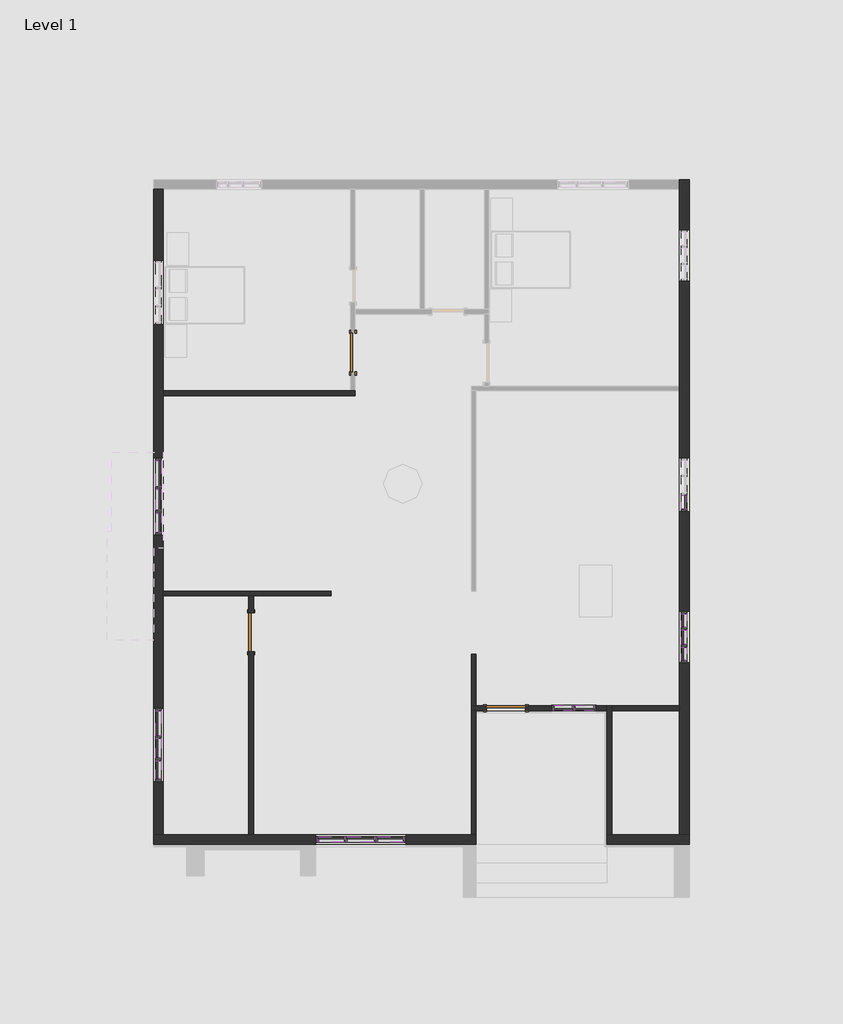
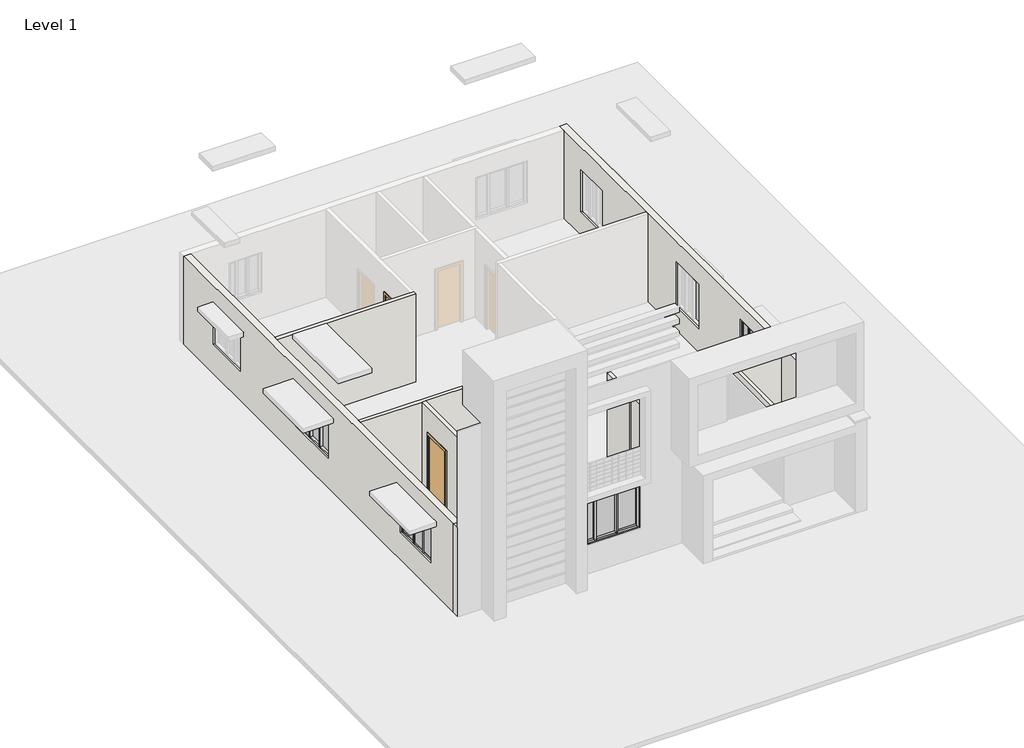
# One storey, part 1 of 2: 49 members, 15 plates, 12 walls, 3 doors.
"""IFC4 building model written with IfcOpenShell, lengths in millimetres."""

from ifc_helpers import new_model, si_unit, frame, origin, origin_with_axes, place, context, project, spatial, polyline, outline, extrude, faceted_brep, transform, mapped, element, save
from components import door_e5f9f3c4, door_305aa2a5, member_3f0e0172, member_ccb4fae7, member_c8b03bc0, member_5215b92c, member_6fb4a552, member_33acc223, member_52eebb51, member_ff1b7d8f, member_5ad95953, member_0c6ed757, member_e9b380b6, member_ff9f2d30, member_6edf370a, member_2ebf4a73, member_5535eeb3, member_1bb00157, member_09480567, member_6b13c281, member_40cdec31, member_e5d39754, member_141a309f, member_b9522cbe, system_panel_glazed_c2bb5d5a, system_panel_glazed_5fa6f1c3, system_panel_glazed_0e598201, system_panel_glazed_cd521809, system_panel_glazed_8f6bde40, system_panel_glazed_4b443884, system_panel_glazed_e0225be8, system_panel_glazed_dc961f7d, system_panel_glazed_14b3f2be, system_panel_glazed_cae65973, system_panel_glazed_06506daa, system_panel_glazed_4e802334

model = new_model("IFC4")

# Units and contexts
model_context = context("Model", 3, world=origin())
ifc_project = project(units=[si_unit("LENGTHUNIT", "METRE", prefix="MILLI")], contexts=[model_context])

# Site, building, storey
site = spatial("IfcSite", under=ifc_project)
building = spatial("IfcBuilding", under=site)
storey = spatial("IfcBuildingStorey", under=building, Name="Level 1", Elevation=0.0)

# Doors
placement = place(None, origin())
door_shape = door_e5f9f3c4(model_context)
element("IfcDoor", 1, ObjectType="Single-Flush : 36\" x 84\"", at=placement, inside=storey, context=model_context, shape_type="MappedRepresentation", body=[
    mapped(door_shape, transform((-18760.1886697, -593.6761954, 0.0), x_axis=(0.0, 1.0, 0.0), y_axis=(-1.0, 0.0, 0.0), z_axis=(0.0, 0.0, 1.0))),
])
element("IfcDoor", 2, ObjectType="Single-Flush : 36\" x 84\"", at=placement, inside=storey, context=model_context, shape_type="MappedRepresentation", body=[
    mapped(door_shape, transform((-21160.4886697, -7194.5011954, 0.0), x_axis=(0.0, 1.0, 0.0), y_axis=(-1.0, 0.0, 0.0), z_axis=(0.0, 0.0, 1.0))),
])
door_2_shape = door_305aa2a5(model_context)
element("IfcDoor", 3, ObjectType="Single-Flush : 36\" x 84\"", at=placement, inside=storey, context=model_context, shape_type="MappedRepresentation", body=[
    mapped(door_2_shape, transform((-15140.6886697, -8985.2011954, 508.0), x_axis=(-1.0, 0.0, 0.0), y_axis=(0.0, -1.0, 0.0), z_axis=(0.0, 0.0, 1.0))),
])

# Members
member_shape = member_3f0e0172(model_context)
element("IfcMember", 4, ObjectType="Rectangular Mullion : 2.5\" x 5\" rectangular", at=placement, inside=storey, context=model_context, shape_type="MappedRepresentation", body=[
    mapped(member_shape, transform((-18957.0386697, -12090.3511954, 2639.2310444), x_axis=(0.0, 0.0, 1.0), y_axis=(0.0, -1.0, 0.0), z_axis=(1.0, 0.0, 0.0))),
])
element("IfcMember", 5, ObjectType="Rectangular Mullion : 2.5\" x 5\" rectangular", at=placement, inside=storey, context=model_context, shape_type="MappedRepresentation", body=[
    mapped(member_shape, transform((-17566.3886697, -12090.3511954, 2639.2310444), x_axis=(0.0, 0.0, 1.0), y_axis=(0.0, -1.0, 0.0), z_axis=(1.0, 0.0, 0.0))),
])
element("IfcMember", 6, ObjectType="Rectangular Mullion : 2.5\" x 5\" rectangular", at=placement, inside=storey, context=model_context, shape_type="MappedRepresentation", body=[
    mapped(member_shape, transform((-23351.2386697, -3759.1511954, 2430.0392006), x_axis=(0.0, 0.0, 1.0), y_axis=(-1.0, 0.0, 0.0), z_axis=(0.0, -1.0, 0.0))),
])
member_2_shape = member_ccb4fae7(model_context)
element("IfcMember", 7, ObjectType="Rectangular Mullion : 2.5\" x 5\" rectangular", at=placement, inside=storey, context=model_context, shape_type="MappedRepresentation", body=[
    mapped(member_2_shape, transform((-18925.2886697, -12090.3511954, 979.2186595), x_axis=(1.0, 0.0, 0.0), y_axis=(0.0, -1.0, 0.0), z_axis=(0.0, 0.0, -1.0))),
])
element("IfcMember", 8, ObjectType="Rectangular Mullion : 2.5\" x 5\" rectangular", at=placement, inside=storey, context=model_context, shape_type="MappedRepresentation", body=[
    mapped(member_2_shape, transform((-18214.0886697, -12090.3511954, 979.2186595), x_axis=(1.0, 0.0, 0.0), y_axis=(0.0, -1.0, 0.0), z_axis=(0.0, 0.0, -1.0))),
])
element("IfcMember", 9, ObjectType="Rectangular Mullion : 2.5\" x 5\" rectangular", at=placement, inside=storey, context=model_context, shape_type="MappedRepresentation", body=[
    mapped(member_shape, transform((-18182.3386697, -12090.3511954, 979.2186595), x_axis=(0.0, 0.0, -1.0), y_axis=(0.0, -1.0, 0.0), z_axis=(-1.0, 0.0, 0.0))),
])
element("IfcMember", 10, ObjectType="Rectangular Mullion : 2.5\" x 5\" rectangular", at=placement, inside=storey, context=model_context, shape_type="MappedRepresentation", body=[
    mapped(member_shape, transform((-19572.9886697, -12090.3511954, 979.2186595), x_axis=(0.0, 0.0, -1.0), y_axis=(0.0, -1.0, 0.0), z_axis=(-1.0, 0.0, 0.0))),
])
element("IfcMember", 11, ObjectType="Rectangular Mullion : 2.5\" x 5\" rectangular", at=placement, inside=storey, context=model_context, shape_type="MappedRepresentation", body=[
    mapped(member_shape, transform((-23351.2386697, -3143.2011954, 1028.1892523), x_axis=(0.0, 0.0, -1.0), y_axis=(-1.0, 0.0, 0.0), z_axis=(0.0, 1.0, 0.0))),
])
member_3_shape = member_c8b03bc0(model_context)
element("IfcMember", 12, ObjectType="Rectangular Mullion : 2.5\" x 5\" rectangular", at=placement, inside=storey, context=model_context, shape_type="MappedRepresentation", body=[
    mapped(member_3_shape, transform((-19636.4886697, -12090.3511954, 2639.2310444), x_axis=(-1.0, 0.0, 0.0), y_axis=(0.0, -1.0, 0.0), z_axis=(0.0, 0.0, 1.0))),
])
element("IfcMember", 13, ObjectType="Rectangular Mullion : 2.5\" x 5\" rectangular", at=placement, inside=storey, context=model_context, shape_type="MappedRepresentation", body=[
    mapped(member_3_shape, transform((-17502.8886697, -12090.3511954, 979.2186595), x_axis=(1.0, 0.0, 0.0), y_axis=(0.0, -1.0, 0.0), z_axis=(0.0, 0.0, -1.0))),
])
member_4_shape = member_5215b92c(model_context)
element("IfcMember", 14, ObjectType="Rectangular Mullion : 2.5\" x 5\" rectangular", at=placement, inside=storey, context=model_context, shape_type="MappedRepresentation", body=[
    mapped(member_4_shape, transform((-18245.8386697, -12090.3511954, 2639.2310444), x_axis=(0.0, 0.0, 1.0), y_axis=(0.0, -1.0, 0.0), z_axis=(1.0, 0.0, 0.0))),
])
element("IfcMember", 15, ObjectType="Rectangular Mullion : 2.5\" x 5\" rectangular", at=placement, inside=storey, context=model_context, shape_type="MappedRepresentation", body=[
    mapped(member_4_shape, transform((-18893.5386697, -12090.3511954, 979.2186595), x_axis=(0.0, 0.0, -1.0), y_axis=(0.0, -1.0, 0.0), z_axis=(-1.0, 0.0, 0.0))),
])
member_5_shape = member_6fb4a552(model_context)
element("IfcMember", 16, ObjectType="Rectangular Mullion : 2.5\" x 5\" rectangular", at=placement, inside=storey, context=model_context, shape_type="MappedRepresentation", body=[
    mapped(member_5_shape, transform((-13508.7386697, -8985.2011954, 2654.6691591), x_axis=(0.0, 0.0, 1.0), y_axis=(0.0, 1.0, 0.0), z_axis=(-1.0, 0.0, 0.0))),
])
element("IfcMember", 17, ObjectType="Rectangular Mullion : 2.5\" x 5\" rectangular", at=placement, inside=storey, context=model_context, shape_type="MappedRepresentation", body=[
    mapped(member_5_shape, transform((-14010.3886697, -8985.2011954, 2654.6691591), x_axis=(0.0, 0.0, 1.0), y_axis=(0.0, 1.0, 0.0), z_axis=(-1.0, 0.0, 0.0))),
])
member_6_shape = member_33acc223(model_context)
element("IfcMember", 18, ObjectType="Rectangular Mullion : 2.5\" x 5\" rectangular", at=placement, inside=storey, context=model_context, shape_type="MappedRepresentation", body=[
    mapped(member_6_shape, transform((-13540.4886697, -8985.2011954, 765.4915318), x_axis=(-1.0, 0.0, 0.0), y_axis=(0.0, 1.0, 0.0), z_axis=(0.0, 0.0, -1.0))),
])
element("IfcMember", 19, ObjectType="Rectangular Mullion : 2.5\" x 5\" rectangular", at=placement, inside=storey, context=model_context, shape_type="MappedRepresentation", body=[
    mapped(member_5_shape, transform((-13572.2386697, -8985.2011954, 765.4915318), x_axis=(0.0, 0.0, -1.0), y_axis=(0.0, 1.0, 0.0), z_axis=(1.0, 0.0, 0.0))),
])
element("IfcMember", 20, ObjectType="Rectangular Mullion : 2.5\" x 5\" rectangular", at=placement, inside=storey, context=model_context, shape_type="MappedRepresentation", body=[
    mapped(member_5_shape, transform((-13070.5886697, -8985.2011954, 765.4915318), x_axis=(0.0, 0.0, -1.0), y_axis=(0.0, 1.0, 0.0), z_axis=(1.0, 0.0, 0.0))),
])
member_7_shape = member_52eebb51(model_context)
element("IfcMember", 21, ObjectType="Rectangular Mullion : 2.5\" x 5\" rectangular", at=placement, inside=storey, context=model_context, shape_type="MappedRepresentation", body=[
    mapped(member_7_shape, transform((-14073.8886697, -8985.2011954, 765.4915318), x_axis=(-1.0, 0.0, 0.0), y_axis=(0.0, 1.0, 0.0), z_axis=(0.0, 0.0, -1.0))),
])
element("IfcMember", 22, ObjectType="Rectangular Mullion : 2.5\" x 5\" rectangular", at=placement, inside=storey, context=model_context, shape_type="MappedRepresentation", body=[
    mapped(member_7_shape, transform((-13007.0886697, -8985.2011954, 2654.6691591), x_axis=(1.0, 0.0, 0.0), y_axis=(0.0, 1.0, 0.0), z_axis=(0.0, 0.0, 1.0))),
])
member_8_shape = member_ff1b7d8f(model_context)
element("IfcMember", 23, ObjectType="Rectangular Mullion : 2.5\" x 5\" rectangular", at=placement, inside=storey, context=model_context, shape_type="MappedRepresentation", body=[
    mapped(member_8_shape, transform((-10930.6386697, -7137.3511954, 2556.4176523), x_axis=(0.0, 0.0, 1.0), y_axis=(1.0, 0.0, 0.0), z_axis=(0.0, 1.0, 0.0))),
])
member_9_shape = member_5ad95953(model_context)
element("IfcMember", 24, ObjectType="Rectangular Mullion : 2.5\" x 5\" rectangular", at=placement, inside=storey, context=model_context, shape_type="MappedRepresentation", body=[
    mapped(member_9_shape, transform((-10930.6386697, -7543.7511954, 2556.4176523), x_axis=(0.0, 0.0, 1.0), y_axis=(1.0, 0.0, 0.0), z_axis=(0.0, 1.0, 0.0))),
])
element("IfcMember", 25, ObjectType="Rectangular Mullion : 2.5\" x 5\" rectangular", at=placement, inside=storey, context=model_context, shape_type="MappedRepresentation", body=[
    mapped(member_9_shape, transform((-10930.6386697, -6762.7011954, 2556.4176523), x_axis=(0.0, 0.0, 1.0), y_axis=(1.0, 0.0, 0.0), z_axis=(0.0, 1.0, 0.0))),
])
member_10_shape = member_0c6ed757(model_context)
element("IfcMember", 26, ObjectType="Rectangular Mullion : 2.5\" x 5\" rectangular", at=placement, inside=storey, context=model_context, shape_type="MappedRepresentation", body=[
    mapped(member_10_shape, transform((-10930.6386697, -7512.0011954, 877.6080724), x_axis=(0.0, 1.0, 0.0), y_axis=(1.0, 0.0, 0.0), z_axis=(0.0, 0.0, -1.0))),
])
element("IfcMember", 27, ObjectType="Rectangular Mullion : 2.5\" x 5\" rectangular", at=placement, inside=storey, context=model_context, shape_type="MappedRepresentation", body=[
    mapped(member_10_shape, transform((-10930.6386697, -7105.6011954, 877.6080724), x_axis=(0.0, 1.0, 0.0), y_axis=(1.0, 0.0, 0.0), z_axis=(0.0, 0.0, -1.0))),
])
element("IfcMember", 28, ObjectType="Rectangular Mullion : 2.5\" x 5\" rectangular", at=placement, inside=storey, context=model_context, shape_type="MappedRepresentation", body=[
    mapped(member_9_shape, transform((-10930.6386697, -7073.8511954, 877.6080724), x_axis=(0.0, 0.0, -1.0), y_axis=(1.0, 0.0, 0.0), z_axis=(0.0, -1.0, 0.0))),
])
element("IfcMember", 29, ObjectType="Rectangular Mullion : 2.5\" x 5\" rectangular", at=placement, inside=storey, context=model_context, shape_type="MappedRepresentation", body=[
    mapped(member_9_shape, transform((-10930.6386697, -7854.9011954, 877.6080724), x_axis=(0.0, 0.0, -1.0), y_axis=(1.0, 0.0, 0.0), z_axis=(0.0, -1.0, 0.0))),
])
element("IfcMember", 30, ObjectType="Rectangular Mullion : 2.5\" x 5\" rectangular", at=placement, inside=storey, context=model_context, shape_type="MappedRepresentation", body=[
    mapped(member_8_shape, transform((-10930.6386697, -7480.2511954, 877.6080724), x_axis=(0.0, 0.0, -1.0), y_axis=(1.0, 0.0, 0.0), z_axis=(0.0, -1.0, 0.0))),
])
member_11_shape = member_e9b380b6(model_context)
element("IfcMember", 31, ObjectType="Rectangular Mullion : 2.5\" x 5\" rectangular", at=placement, inside=storey, context=model_context, shape_type="MappedRepresentation", body=[
    mapped(member_11_shape, transform((-10930.6386697, -6699.2011954, 877.6080724), x_axis=(0.0, 1.0, 0.0), y_axis=(1.0, 0.0, 0.0), z_axis=(0.0, 0.0, -1.0))),
])
element("IfcMember", 32, ObjectType="Rectangular Mullion : 2.5\" x 5\" rectangular", at=placement, inside=storey, context=model_context, shape_type="MappedRepresentation", body=[
    mapped(member_11_shape, transform((-10930.6386697, -7918.4011954, 2556.4176523), x_axis=(0.0, -1.0, 0.0), y_axis=(1.0, 0.0, 0.0), z_axis=(0.0, 0.0, 1.0))),
])
member_12_shape = member_ff9f2d30(model_context)
element("IfcMember", 33, ObjectType="Rectangular Mullion : 2.5\" x 5\" rectangular", at=placement, inside=storey, context=model_context, shape_type="MappedRepresentation", body=[
    mapped(member_12_shape, transform((-10930.6386697, -4292.5511954, 2353.4996799), x_axis=(0.0, 0.0, 1.0), y_axis=(-1.0, 0.0, 0.0), z_axis=(0.0, -1.0, 0.0))),
])
member_13_shape = member_6edf370a(model_context)
element("IfcMember", 34, ObjectType="Rectangular Mullion : 2.5\" x 5\" rectangular", at=placement, inside=storey, context=model_context, shape_type="MappedRepresentation", body=[
    mapped(member_13_shape, transform((-10930.6386697, -4356.0511954, 821.4712655), x_axis=(0.0, -1.0, 0.0), y_axis=(-1.0, 0.0, 0.0), z_axis=(0.0, 0.0, -1.0))),
])
member_14_shape = member_2ebf4a73(model_context)
element("IfcMember", 35, ObjectType="Rectangular Mullion : 2.5\" x 5\" rectangular", at=placement, inside=storey, context=model_context, shape_type="MappedRepresentation", body=[
    mapped(member_14_shape, transform((-23351.2386697, -4317.9511954, 2430.0392006), x_axis=(0.0, 0.0, 1.0), y_axis=(-1.0, 0.0, 0.0), z_axis=(0.0, -1.0, 0.0))),
])
member_15_shape = member_5535eeb3(model_context)
element("IfcMember", 36, ObjectType="Rectangular Mullion : 2.5\" x 5\" rectangular", at=placement, inside=storey, context=model_context, shape_type="MappedRepresentation", body=[
    mapped(member_15_shape, transform((-23351.2386697, -4845.0011954, 2430.0392006), x_axis=(0.0, 0.0, 1.0), y_axis=(-1.0, 0.0, 0.0), z_axis=(0.0, -1.0, 0.0))),
])
member_16_shape = member_1bb00157(model_context)
element("IfcMember", 37, ObjectType="Rectangular Mullion : 2.5\" x 5\" rectangular", at=placement, inside=storey, context=model_context, shape_type="MappedRepresentation", body=[
    mapped(member_16_shape, transform((-23351.2386697, -3790.9011954, 1028.1892523), x_axis=(0.0, -1.0, 0.0), y_axis=(-1.0, 0.0, 0.0), z_axis=(0.0, 0.0, -1.0))),
])
element("IfcMember", 38, ObjectType="Rectangular Mullion : 2.5\" x 5\" rectangular", at=placement, inside=storey, context=model_context, shape_type="MappedRepresentation", body=[
    mapped(member_16_shape, transform((-23351.2386697, -4349.7011954, 1028.1892523), x_axis=(0.0, -1.0, 0.0), y_axis=(-1.0, 0.0, 0.0), z_axis=(0.0, 0.0, -1.0))),
])
element("IfcMember", 39, ObjectType="Rectangular Mullion : 2.5\" x 5\" rectangular", at=placement, inside=storey, context=model_context, shape_type="MappedRepresentation", body=[
    mapped(member_15_shape, transform((-23351.2386697, -4381.4511954, 1028.1892523), x_axis=(0.0, 0.0, -1.0), y_axis=(-1.0, 0.0, 0.0), z_axis=(0.0, 1.0, 0.0))),
])
element("IfcMember", 40, ObjectType="Rectangular Mullion : 2.5\" x 5\" rectangular", at=placement, inside=storey, context=model_context, shape_type="MappedRepresentation", body=[
    mapped(member_14_shape, transform((-23351.2386697, -3822.6511954, 1028.1892523), x_axis=(0.0, 0.0, -1.0), y_axis=(-1.0, 0.0, 0.0), z_axis=(0.0, 1.0, 0.0))),
])
member_17_shape = member_09480567(model_context)
element("IfcMember", 41, ObjectType="Rectangular Mullion : 2.5\" x 5\" rectangular", at=placement, inside=storey, context=model_context, shape_type="MappedRepresentation", body=[
    mapped(member_17_shape, transform((-23351.2386697, -4908.5011954, 1028.1892523), x_axis=(0.0, -1.0, 0.0), y_axis=(-1.0, 0.0, 0.0), z_axis=(0.0, 0.0, -1.0))),
])
element("IfcMember", 42, ObjectType="Rectangular Mullion : 2.5\" x 5\" rectangular", at=placement, inside=storey, context=model_context, shape_type="MappedRepresentation", body=[
    mapped(member_17_shape, transform((-23351.2386697, -3079.7011954, 2430.0392006), x_axis=(0.0, 1.0, 0.0), y_axis=(-1.0, 0.0, 0.0), z_axis=(0.0, 0.0, 1.0))),
])
member_18_shape = member_6b13c281(model_context)
element("IfcMember", 43, ObjectType="Rectangular Mullion : 2.5\" x 5\" rectangular", at=placement, inside=storey, context=model_context, shape_type="MappedRepresentation", body=[
    mapped(member_18_shape, transform((-23351.2386697, -10226.6261954, 2393.4159661), x_axis=(0.0, 0.0, 1.0), y_axis=(1.0, 0.0, 0.0), z_axis=(0.0, 1.0, 0.0))),
])
member_19_shape = member_40cdec31(model_context)
element("IfcMember", 44, ObjectType="Rectangular Mullion : 2.5\" x 5\" rectangular", at=placement, inside=storey, context=model_context, shape_type="MappedRepresentation", body=[
    mapped(member_19_shape, transform((-23351.2386697, -9702.7511954, 2393.4159661), x_axis=(0.0, 0.0, 1.0), y_axis=(1.0, 0.0, 0.0), z_axis=(0.0, 1.0, 0.0))),
])
member_20_shape = member_e5d39754(model_context)
element("IfcMember", 45, ObjectType="Rectangular Mullion : 2.5\" x 5\" rectangular", at=placement, inside=storey, context=model_context, shape_type="MappedRepresentation", body=[
    mapped(member_20_shape, transform((-23351.2386697, -9048.7011954, 2393.4159661), x_axis=(0.0, 0.0, 1.0), y_axis=(1.0, 0.0, 0.0), z_axis=(0.0, 1.0, 0.0))),
])
member_21_shape = member_141a309f(model_context)
element("IfcMember", 46, ObjectType="Rectangular Mullion : 2.5\" x 5\" rectangular", at=placement, inside=storey, context=model_context, shape_type="MappedRepresentation", body=[
    mapped(member_21_shape, transform((-23351.2386697, -9671.0011954, 940.8966177), x_axis=(0.0, 1.0, 0.0), y_axis=(1.0, 0.0, 0.0), z_axis=(0.0, 0.0, -1.0))),
])
element("IfcMember", 47, ObjectType="Rectangular Mullion : 2.5\" x 5\" rectangular", at=placement, inside=storey, context=model_context, shape_type="MappedRepresentation", body=[
    mapped(member_21_shape, transform((-23351.2386697, -10194.8761954, 940.8966177), x_axis=(0.0, 1.0, 0.0), y_axis=(1.0, 0.0, 0.0), z_axis=(0.0, 0.0, -1.0))),
])
element("IfcMember", 48, ObjectType="Rectangular Mullion : 2.5\" x 5\" rectangular", at=placement, inside=storey, context=model_context, shape_type="MappedRepresentation", body=[
    mapped(member_19_shape, transform((-23351.2386697, -10163.1261954, 940.8966177), x_axis=(0.0, 0.0, -1.0), y_axis=(1.0, 0.0, 0.0), z_axis=(0.0, -1.0, 0.0))),
])
element("IfcMember", 49, ObjectType="Rectangular Mullion : 2.5\" x 5\" rectangular", at=placement, inside=storey, context=model_context, shape_type="MappedRepresentation", body=[
    mapped(member_20_shape, transform((-23351.2386697, -9639.2511954, 940.8966177), x_axis=(0.0, 0.0, -1.0), y_axis=(1.0, 0.0, 0.0), z_axis=(0.0, -1.0, 0.0))),
])
element("IfcMember", 50, ObjectType="Rectangular Mullion : 2.5\" x 5\" rectangular", at=placement, inside=storey, context=model_context, shape_type="MappedRepresentation", body=[
    mapped(member_18_shape, transform((-23351.2386697, -10655.2511954, 940.8966177), x_axis=(0.0, 0.0, -1.0), y_axis=(1.0, 0.0, 0.0), z_axis=(0.0, -1.0, 0.0))),
])
member_22_shape = member_b9522cbe(model_context)
element("IfcMember", 51, ObjectType="Rectangular Mullion : 2.5\" x 5\" rectangular", at=placement, inside=storey, context=model_context, shape_type="MappedRepresentation", body=[
    mapped(member_22_shape, transform((-23351.2386697, -10718.7511954, 2393.4159661), x_axis=(0.0, -1.0, 0.0), y_axis=(1.0, 0.0, 0.0), z_axis=(0.0, 0.0, 1.0))),
])
element("IfcMember", 52, ObjectType="Rectangular Mullion : 2.5\" x 5\" rectangular", at=placement, inside=storey, context=model_context, shape_type="MappedRepresentation", body=[
    mapped(member_22_shape, transform((-23351.2386697, -8985.2011954, 940.8966177), x_axis=(0.0, 1.0, 0.0), y_axis=(1.0, 0.0, 0.0), z_axis=(0.0, 0.0, -1.0))),
])

# Plates
system_panel_glazed_shape = system_panel_glazed_c2bb5d5a(model_context)
element("IfcPlate", 53, ObjectType="System Panel : Glazed", at=placement, inside=storey, context=model_context, shape_type="MappedRepresentation", body=[
    mapped(system_panel_glazed_shape, transform((-19265.0136697, -12090.3511954, 1042.7186595), x_axis=(1.0, 0.0, 0.0), y_axis=(0.0, 1.0, 0.0), z_axis=(0.0, 0.0, 1.0))),
])
element("IfcPlate", 54, ObjectType="System Panel : Glazed", at=placement, inside=storey, context=model_context, shape_type="MappedRepresentation", body=[
    mapped(system_panel_glazed_shape, transform((-17874.3636697, -12090.3511954, 1042.7186595), x_axis=(1.0, 0.0, 0.0), y_axis=(0.0, 1.0, 0.0), z_axis=(0.0, 0.0, 1.0))),
])
system_panel_glazed_2_shape = system_panel_glazed_5fa6f1c3(model_context)
element("IfcPlate", 55, ObjectType="System Panel : Glazed", at=placement, inside=storey, context=model_context, shape_type="MappedRepresentation", body=[
    mapped(system_panel_glazed_2_shape, transform((-18569.6886697, -12090.3511954, 1042.7186595), x_axis=(1.0, 0.0, 0.0), y_axis=(0.0, 1.0, 0.0), z_axis=(0.0, 0.0, 1.0))),
])
system_panel_glazed_3_shape = system_panel_glazed_0e598201(model_context)
element("IfcPlate", 56, ObjectType="System Panel : Glazed", at=placement, inside=storey, context=model_context, shape_type="MappedRepresentation", body=[
    mapped(system_panel_glazed_3_shape, transform((-13289.6636697, -8985.2011954, 828.9915318), x_axis=(-1.0, 0.0, 0.0), y_axis=(0.0, -1.0, 0.0), z_axis=(0.0, 0.0, 1.0))),
])
element("IfcPlate", 57, ObjectType="System Panel : Glazed", at=placement, inside=storey, context=model_context, shape_type="MappedRepresentation", body=[
    mapped(system_panel_glazed_3_shape, transform((-13791.3136697, -8985.2011954, 828.9915318), x_axis=(-1.0, 0.0, 0.0), y_axis=(0.0, -1.0, 0.0), z_axis=(0.0, 0.0, 1.0))),
])
system_panel_glazed_4_shape = system_panel_glazed_cd521809(model_context)
element("IfcPlate", 58, ObjectType="System Panel : Glazed", at=placement, inside=storey, context=model_context, shape_type="MappedRepresentation", body=[
    mapped(system_panel_glazed_4_shape, transform((-10930.6386697, -7308.8011954, 941.1080724), x_axis=(0.0, 1.0, 0.0), y_axis=(-1.0, 0.0, 0.0), z_axis=(0.0, 0.0, 1.0))),
])
system_panel_glazed_5_shape = system_panel_glazed_8f6bde40(model_context)
element("IfcPlate", 59, ObjectType="System Panel : Glazed", at=placement, inside=storey, context=model_context, shape_type="MappedRepresentation", body=[
    mapped(system_panel_glazed_5_shape, transform((-10930.6386697, -7699.3261954, 941.1080724), x_axis=(0.0, 1.0, 0.0), y_axis=(-1.0, 0.0, 0.0), z_axis=(0.0, 0.0, 1.0))),
])
element("IfcPlate", 60, ObjectType="System Panel : Glazed", at=placement, inside=storey, context=model_context, shape_type="MappedRepresentation", body=[
    mapped(system_panel_glazed_5_shape, transform((-10930.6386697, -6918.2761954, 941.1080724), x_axis=(0.0, 1.0, 0.0), y_axis=(-1.0, 0.0, 0.0), z_axis=(0.0, 0.0, 1.0))),
])
system_panel_glazed_6_shape = system_panel_glazed_4b443884(model_context)
element("IfcPlate", 61, ObjectType="System Panel : Glazed", at=placement, inside=storey, context=model_context, shape_type="MappedRepresentation", body=[
    mapped(system_panel_glazed_6_shape, transform((-10930.6386697, -4127.4511954, 884.9712655), x_axis=(0.0, -1.0, 0.0), y_axis=(1.0, 0.0, 0.0), z_axis=(0.0, 0.0, 1.0))),
])
system_panel_glazed_7_shape = system_panel_glazed_e0225be8(model_context)
element("IfcPlate", 62, ObjectType="System Panel : Glazed", at=placement, inside=storey, context=model_context, shape_type="MappedRepresentation", body=[
    mapped(system_panel_glazed_7_shape, transform((-23351.2386697, -3451.1761954, 1091.6892523), x_axis=(0.0, -1.0, 0.0), y_axis=(1.0, 0.0, 0.0), z_axis=(0.0, 0.0, 1.0))),
])
system_panel_glazed_8_shape = system_panel_glazed_dc961f7d(model_context)
element("IfcPlate", 63, ObjectType="System Panel : Glazed", at=placement, inside=storey, context=model_context, shape_type="MappedRepresentation", body=[
    mapped(system_panel_glazed_8_shape, transform((-23351.2386697, -4070.3011954, 1091.6892523), x_axis=(0.0, -1.0, 0.0), y_axis=(1.0, 0.0, 0.0), z_axis=(0.0, 0.0, 1.0))),
])
system_panel_glazed_9_shape = system_panel_glazed_14b3f2be(model_context)
element("IfcPlate", 64, ObjectType="System Panel : Glazed", at=placement, inside=storey, context=model_context, shape_type="MappedRepresentation", body=[
    mapped(system_panel_glazed_9_shape, transform((-23351.2386697, -4613.2261954, 1091.6892523), x_axis=(0.0, -1.0, 0.0), y_axis=(1.0, 0.0, 0.0), z_axis=(0.0, 0.0, 1.0))),
])
system_panel_glazed_10_shape = system_panel_glazed_cae65973(model_context)
element("IfcPlate", 65, ObjectType="System Panel : Glazed", at=placement, inside=storey, context=model_context, shape_type="MappedRepresentation", body=[
    mapped(system_panel_glazed_10_shape, transform((-23351.2386697, -10440.9386954, 1004.3966177), x_axis=(0.0, 1.0, 0.0), y_axis=(-1.0, 0.0, 0.0), z_axis=(0.0, 0.0, 1.0))),
])
system_panel_glazed_11_shape = system_panel_glazed_06506daa(model_context)
element("IfcPlate", 66, ObjectType="System Panel : Glazed", at=placement, inside=storey, context=model_context, shape_type="MappedRepresentation", body=[
    mapped(system_panel_glazed_11_shape, transform((-23351.2386697, -9343.9761954, 1004.3966177), x_axis=(0.0, 1.0, 0.0), y_axis=(-1.0, 0.0, 0.0), z_axis=(0.0, 0.0, 1.0))),
])
system_panel_glazed_12_shape = system_panel_glazed_4e802334(model_context)
element("IfcPlate", 67, ObjectType="System Panel : Glazed", at=placement, inside=storey, context=model_context, shape_type="MappedRepresentation", body=[
    mapped(system_panel_glazed_12_shape, transform((-23351.2386697, -9932.9386954, 1004.3966177), x_axis=(0.0, 1.0, 0.0), y_axis=(-1.0, 0.0, 0.0), z_axis=(0.0, 0.0, 1.0))),
])

# Walls
element("IfcWall", 68, ObjectType="4.5\"", at=placement, inside=storey, context=model_context, shape_type="SweptSolid", body=[
    extrude(outline(polyline([(-6337.2511954, 0.0), (-6737.3011954, 0.0), (-6737.3011954, 2133.6), (-7651.7011954, 2133.6), (-7651.7011954, 0.0), (-11976.0511954, 0.0), (-11976.0511954, 3048.0), (-6337.2511954, 3048.0), (-6337.2511954, 0.0)])), frame((-21217.6386697, 0.0, 0.0), z_axis=(1.0, 0.0, 0.0), x_axis=(0.0, 1.0, 0.0)), (0.0, 0.0, 1.0), 114.3),
])
element("IfcWall", 69, ObjectType="4.5\"", at=placement, inside=storey, context=model_context, shape_type="Brep", body=[
    faceted_brep([(-12645.1386697, -11976.0511954, 0.0), (-12645.1386697, -9042.3511954, 0.0), (-12645.1386697, -8928.0511954, 0.0), (-12645.1386697, -8928.0511954, 3048.0), (-12645.1386697, -9042.3511954, 3048.0), (-12645.1386697, -11976.0511954, 3048.0), (-12759.4386697, -11976.0511954, 0.0), (-12759.4386697, -11976.0511954, 3048.0), (-12759.4386697, -9042.3511954, 3048.0), (-12759.4386697, -8928.0511954, 3048.0), (-12759.4386697, -8928.0511954, 0.0), (-12759.4386697, -9042.3511954, 0.0)], [[[0, 1, 2, 3, 4, 5]], [[6, 7, 8, 9, 10, 11]], [[2, 1, 0, 6, 11, 10]], [[5, 4, 3, 9, 8, 7]], [[0, 5, 7, 6]], [[3, 2, 10, 9]]]),
])
element("IfcWall", 70, ObjectType="4.5\"", at=placement, inside=storey, context=model_context, shape_type="SweptSolid", body=[
    extrude(outline(polyline([(-11044.9386697, -9042.3511954), (-12645.1386697, -9042.3511954), (-12645.1386697, -8928.0511954), (-11044.9386697, -8928.0511954), (-11044.9386697, -9042.3511954)])), origin_with_axes(), (0.0, 0.0, 1.0), 3048.0),
])
element("IfcWall", 71, ObjectType="4.5\"", at=placement, inside=storey, context=model_context, shape_type="Brep", body=[
    faceted_brep([(-12759.4386697, -8928.0511954, 0.0), (-15845.5386697, -8928.0511954, 0.0), (-15959.8386697, -8928.0511954, 0.0), (-15959.8386697, -8928.0511954, 3048.0), (-15845.5386697, -8928.0511954, 3048.0), (-12759.4386697, -8928.0511954, 3048.0), (-14683.4886697, -8928.0511954, 508.0), (-14683.4886697, -8928.0511954, 2641.6), (-15597.8886697, -8928.0511954, 2641.6), (-15597.8886697, -8928.0511954, 508.0), (-13007.0886697, -8928.0511954, 765.4915318), (-13007.0886697, -8928.0511954, 2654.6691591), (-14073.8886697, -8928.0511954, 2654.6691591), (-14073.8886697, -8928.0511954, 765.4915318), (-15959.8386697, -9042.3511954, 0.0), (-15845.5386697, -9042.3511954, 0.0), (-12759.4386697, -9042.3511954, 0.0), (-12759.4386697, -9042.3511954, 3048.0), (-15845.5386697, -9042.3511954, 3048.0), (-15959.8386697, -9042.3511954, 3048.0), (-14683.4886697, -9042.3511954, 508.0), (-15597.8886697, -9042.3511954, 508.0), (-15597.8886697, -9042.3511954, 2641.6), (-14683.4886697, -9042.3511954, 2641.6), (-13007.0886697, -9042.3511954, 2654.6691591), (-13007.0886697, -9042.3511954, 765.4915318), (-14073.8886697, -9042.3511954, 765.4915318), (-14073.8886697, -9042.3511954, 2654.6691591)], [[[0, 1, 2, 3, 4, 5], [6, 7, 8, 9], [10, 11, 12, 13]], [[14, 15, 16, 17, 18, 19], [20, 21, 22, 23], [24, 25, 26, 27]], [[2, 1, 0, 16, 15, 14]], [[5, 4, 3, 19, 18, 17]], [[0, 5, 17, 16]], [[3, 2, 14, 19]], [[21, 20, 6, 9]], [[22, 21, 9, 8]], [[23, 22, 8, 7]], [[20, 23, 7, 6]], [[10, 25, 24, 11]], [[11, 24, 27, 12]], [[12, 27, 26, 13]], [[25, 10, 13, 26]]]),
])
element("IfcWall", 72, ObjectType="4.5\"", at=placement, inside=storey, context=model_context, shape_type="SweptSolid", body=[
    extrude(outline(polyline([(-15959.8386697, -11976.0511954), (-15959.8386697, -9042.3511954), (-15845.5386697, -9042.3511954), (-15845.5386697, -11976.0511954), (-15959.8386697, -11976.0511954)])), origin_with_axes(), (0.0, 0.0, 1.0), 3048.0),
])
element("IfcWall", 73, ObjectType="4.5\"", at=placement, inside=storey, context=model_context, shape_type="SweptSolid", body=[
    extrude(outline(polyline([(-15845.5386697, -7708.8511954), (-15845.5386697, -8928.0511954), (-15959.8386697, -8928.0511954), (-15959.8386697, -7708.8511954), (-15845.5386697, -7708.8511954)])), origin_with_axes(), (0.0, 0.0, 1.0), 3048.0),
])
element("IfcWall", 74, ObjectType="4.5\"", at=placement, inside=storey, context=model_context, shape_type="Brep", body=[
    faceted_brep([(-23236.9386697, -1612.8511954, 0.0), (-18703.0386697, -1612.8511954, 0.0), (-18703.0386697, -1612.8511954, 3048.0), (-23236.9386697, -1612.8511954, 3048.0), (-23236.9386697, -1498.5511954, 0.0), (-23236.9386697, -1498.5511954, 3048.0), (-18817.3386697, -1498.5511954, 3048.0), (-18703.0386697, -1498.5511954, 3048.0), (-18703.0386697, -1498.5511954, 0.0), (-18817.3386697, -1498.5511954, 0.0)], [[[0, 1, 2, 3]], [[4, 5, 6, 7, 8, 9]], [[1, 0, 4, 9, 8]], [[3, 2, 7, 6, 5]], [[0, 3, 5, 4]], [[2, 1, 8, 7]]]),
])
element("IfcWall", 75, ObjectType="4.5\"", at=placement, inside=storey, context=model_context, shape_type="Brep", body=[
    faceted_brep([(-23236.9386697, -6337.2511954, 0.0), (-21217.6386697, -6337.2511954, 0.0), (-21103.3386697, -6337.2511954, 0.0), (-19274.5386697, -6337.2511954, 0.0), (-19274.5386697, -6337.2511954, 3048.0), (-21103.3386697, -6337.2511954, 3048.0), (-21217.6386697, -6337.2511954, 3048.0), (-23236.9386697, -6337.2511954, 3048.0), (-23236.9386697, -6222.9511954, 0.0), (-23236.9386697, -6222.9511954, 3048.0), (-19274.5386697, -6222.9511954, 3048.0), (-19274.5386697, -6222.9511954, 0.0)], [[[0, 1, 2, 3, 4, 5, 6, 7]], [[8, 9, 10, 11]], [[3, 2, 1, 0, 8, 11]], [[4, 3, 11, 10]], [[7, 6, 5, 4, 10, 9]], [[0, 7, 9, 8]]]),
])
element("IfcWall", 76, ObjectType="9\"", at=placement, inside=storey, context=model_context, shape_type="Brep", body=[
    faceted_brep([(-23465.5386697, -12204.6511954, 0.0), (-15845.5386697, -12204.6511954, 0.0), (-15845.5386697, -12204.6511954, 3048.0), (-23465.5386697, -12204.6511954, 3048.0), (-19636.4886697, -12204.6511954, 979.2186595), (-19636.4886697, -12204.6511954, 2639.2310444), (-17502.8886697, -12204.6511954, 2639.2310444), (-17502.8886697, -12204.6511954, 979.2186595), (-15845.5386697, -11976.0511954, 0.0), (-15959.8386697, -11976.0511954, 0.0), (-21103.3386697, -11976.0511954, 0.0), (-21217.6386697, -11976.0511954, 0.0), (-23236.9386697, -11976.0511954, 0.0), (-23465.5386697, -11976.0511954, 0.0), (-23465.5386697, -11976.0511954, 3048.0), (-23236.9386697, -11976.0511954, 3048.0), (-21217.6386697, -11976.0511954, 3048.0), (-21103.3386697, -11976.0511954, 3048.0), (-15959.8386697, -11976.0511954, 3048.0), (-15845.5386697, -11976.0511954, 3048.0), (-19636.4886697, -11976.0511954, 2639.2310444), (-19636.4886697, -11976.0511954, 979.2186595), (-17502.8886697, -11976.0511954, 979.2186595), (-17502.8886697, -11976.0511954, 2639.2310444)], [[[0, 1, 2, 3], [4, 5, 6, 7]], [[8, 9, 10, 11, 12, 13, 14, 15, 16, 17, 18, 19], [20, 21, 22, 23]], [[1, 0, 13, 12, 11, 10, 9, 8]], [[2, 1, 8, 19]], [[3, 2, 19, 18, 17, 16, 15, 14]], [[0, 3, 14, 13]], [[4, 21, 20, 5]], [[5, 20, 23, 6]], [[6, 23, 22, 7]], [[21, 4, 7, 22]]]),
])
element("IfcWall", 77, ObjectType="9\"", at=placement, inside=storey, context=model_context, shape_type="Brep", body=[
    faceted_brep([(-10816.3386697, -11976.0511954, 0.0), (-10816.3386697, 3492.5488046, 0.0), (-10816.3386697, 3492.5488046, 3048.0), (-10816.3386697, -11976.0511954, 3048.0), (-10816.3386697, 2311.4488046, 2267.0732017), (-10816.3386697, 2311.4488046, 809.8934331), (-10816.3386697, 1092.2488046, 809.8934331), (-10816.3386697, 1092.2488046, 2267.0732017), (-10816.3386697, -3079.7011954, 2353.4996799), (-10816.3386697, -3079.7011954, 821.4712655), (-10816.3386697, -4356.0511954, 821.4712655), (-10816.3386697, -4356.0511954, 2353.4996799), (-10816.3386697, -7918.4011954, 877.6080724), (-10816.3386697, -7918.4011954, 2556.4176523), (-10816.3386697, -6699.2011954, 2556.4176523), (-10816.3386697, -6699.2011954, 877.6080724), (-11044.9386697, 3492.5488046, 0.0), (-11044.9386697, 3263.9488046, 0.0), (-11044.9386697, -1384.2511954, 0.0), (-11044.9386697, -1498.5511954, 0.0), (-11044.9386697, -8928.0511954, 0.0), (-11044.9386697, -9042.3511954, 0.0), (-11044.9386697, -11976.0511954, 0.0), (-11044.9386697, -11976.0511954, 3048.0), (-11044.9386697, -9042.3511954, 3048.0), (-11044.9386697, -8928.0511954, 3048.0), (-11044.9386697, -1498.5511954, 3048.0), (-11044.9386697, -1384.2511954, 3048.0), (-11044.9386697, 3263.9488046, 3048.0), (-11044.9386697, 3492.5488046, 3048.0), (-11044.9386697, 2311.4488046, 809.8934331), (-11044.9386697, 2311.4488046, 2267.0732017), (-11044.9386697, 1092.2488046, 2267.0732017), (-11044.9386697, 1092.2488046, 809.8934331), (-11044.9386697, -3079.7011954, 821.4712655), (-11044.9386697, -3079.7011954, 2353.4996799), (-11044.9386697, -4356.0511954, 2353.4996799), (-11044.9386697, -4356.0511954, 821.4712655), (-11044.9386697, -7918.4011954, 2556.4176523), (-11044.9386697, -7918.4011954, 877.6080724), (-11044.9386697, -6699.2011954, 877.6080724), (-11044.9386697, -6699.2011954, 2556.4176523)], [[[0, 1, 2, 3], [4, 5, 6, 7], [8, 9, 10, 11], [12, 13, 14, 15]], [[16, 17, 18, 19, 20, 21, 22, 23, 24, 25, 26, 27, 28, 29], [30, 31, 32, 33], [34, 35, 36, 37], [38, 39, 40, 41]], [[1, 0, 22, 21, 20, 19, 18, 17, 16]], [[3, 2, 29, 28, 27, 26, 25, 24, 23]], [[0, 3, 23, 22]], [[2, 1, 16, 29]], [[30, 5, 4, 31]], [[31, 4, 7, 32]], [[32, 7, 6, 33]], [[5, 30, 33, 6]], [[8, 35, 34, 9]], [[35, 8, 11, 36]], [[36, 11, 10, 37]], [[9, 34, 37, 10]], [[38, 13, 12, 39]], [[13, 38, 41, 14]], [[14, 41, 40, 15]], [[39, 12, 15, 40]]]),
])
element("IfcWall", 78, ObjectType="9\"", at=placement, inside=storey, context=model_context, shape_type="Brep", body=[
    faceted_brep([(-23465.5386697, 3263.9488046, 0.0), (-23465.5386697, -11976.0511954, 0.0), (-23465.5386697, -11976.0511954, 3048.0), (-23465.5386697, 3263.9488046, 3048.0), (-23465.5386697, 1587.5488046, 1017.4338808), (-23465.5386697, 1587.5488046, 2332.8596388), (-23465.5386697, 63.5488046, 2332.8596388), (-23465.5386697, 63.5488046, 1017.4338808), (-23465.5386697, -3079.7011954, 1028.1892523), (-23465.5386697, -3079.7011954, 2430.0392006), (-23465.5386697, -4908.5011954, 2430.0392006), (-23465.5386697, -4908.5011954, 1028.1892523), (-23465.5386697, -10718.7511954, 2393.4159661), (-23465.5386697, -10718.7511954, 940.8966177), (-23465.5386697, -8985.2011954, 940.8966177), (-23465.5386697, -8985.2011954, 2393.4159661), (-23236.9386697, -11976.0511954, 0.0), (-23236.9386697, -6337.2511954, 0.0), (-23236.9386697, -6222.9511954, 0.0), (-23236.9386697, -1612.8511954, 0.0), (-23236.9386697, -1498.5511954, 0.0), (-23236.9386697, 3263.9488046, 0.0), (-23236.9386697, 3263.9488046, 3048.0), (-23236.9386697, -1498.5511954, 3048.0), (-23236.9386697, -1612.8511954, 3048.0), (-23236.9386697, -6222.9511954, 3048.0), (-23236.9386697, -6337.2511954, 3048.0), (-23236.9386697, -11976.0511954, 3048.0), (-23236.9386697, 1587.5488046, 2332.8596388), (-23236.9386697, 1587.5488046, 1017.4338808), (-23236.9386697, 63.5488046, 1017.4338808), (-23236.9386697, 63.5488046, 2332.8596388), (-23236.9386697, -3079.7011954, 2430.0392006), (-23236.9386697, -3079.7011954, 1028.1892523), (-23236.9386697, -4908.5011954, 1028.1892523), (-23236.9386697, -4908.5011954, 2430.0392006), (-23236.9386697, -10718.7511954, 940.8966177), (-23236.9386697, -10718.7511954, 2393.4159661), (-23236.9386697, -8985.2011954, 2393.4159661), (-23236.9386697, -8985.2011954, 940.8966177)], [[[0, 1, 2, 3], [4, 5, 6, 7], [8, 9, 10, 11], [12, 13, 14, 15]], [[16, 17, 18, 19, 20, 21, 22, 23, 24, 25, 26, 27], [28, 29, 30, 31], [32, 33, 34, 35], [36, 37, 38, 39]], [[1, 0, 21, 20, 19, 18, 17, 16]], [[3, 2, 27, 26, 25, 24, 23, 22]], [[0, 3, 22, 21]], [[2, 1, 16, 27]], [[28, 5, 4, 29]], [[5, 28, 31, 6]], [[6, 31, 30, 7]], [[29, 4, 7, 30]], [[8, 33, 32, 9]], [[9, 32, 35, 10]], [[34, 11, 10, 35]], [[33, 8, 11, 34]], [[36, 13, 12, 37]], [[37, 12, 15, 38]], [[38, 15, 14, 39]], [[13, 36, 39, 14]]]),
])
element("IfcWall", 79, ObjectType="9\"", at=placement, inside=storey, context=model_context, shape_type="Brep", body=[
    faceted_brep([(-12759.4386697, -12204.6511954, 0.0), (-10816.3386697, -12204.6511954, 0.0), (-10816.3386697, -12204.6511954, 3048.0), (-12759.4386697, -12204.6511954, 3048.0), (-12759.4386697, -11976.0511954, 0.0), (-12759.4386697, -11976.0511954, 3048.0), (-12645.1386697, -11976.0511954, 3048.0), (-11044.9386697, -11976.0511954, 3048.0), (-10816.3386697, -11976.0511954, 3048.0), (-10816.3386697, -11976.0511954, 0.0), (-11044.9386697, -11976.0511954, 0.0), (-12645.1386697, -11976.0511954, 0.0)], [[[0, 1, 2, 3]], [[4, 5, 6, 7, 8, 9, 10, 11]], [[1, 0, 4, 11, 10, 9]], [[3, 2, 8, 7, 6, 5]], [[0, 3, 5, 4]], [[2, 1, 9, 8]]]),
])

save(model, "model.ifc")

# Revit data of these elements
# Type "Single-Flush : 36\" x 84\""
#   Type Mark = "1"
#   Construction Type Id = "MDOOR"
#   Assembly Code = "C1020"
#   Analytic Construction = "Metal"
#   Thickness = 0' - 2"
#   Heat Transfer Coefficient (U) = 0.651978 BTU/(h·ft²·°F)
#   Height = 7' - 0"
#   Trim Projection Ext = 0' - 1"
#   Trim Projection Int = 0' - 1"
#   Trim Width = 0' - 3"
#   Width = 3' - 0"
#   Define Thermal Properties by = 1
#   Define Thermal Properties by = 1
#   Door Material = Door - Panel
#   Frame Material = Door - Frame
#   Visual Light Transmittance = 0
#   Solar Heat Gain Coefficient = 0
#   Function = (empty or 0)
#   Wall Closure = (empty or 0)
# Type "Rectangular Mullion : 2.5\" x 5\" rectangular"
#   built-in parameter 1007304 = 0.416667 (stored number, unit not read)
#   built-in parameter 1007301 = 0.104167 (stored number, unit not read)
#   built-in parameter 1007300 = 0.104167 (stored number, unit not read)
# Type "System Panel : Glazed"
#   Construction Type Id = "GSP4R"
#   Analytic Construction = "1/8 in Pilkington single glazing"
#   Visual Light Transmittance = 0.9
#   Solar Heat Gain Coefficient = 0.86
#   Heat Transfer Coefficient (U) = 1.18115 BTU/(h·ft²·°F)
#   Define Thermal Properties by = 1
# Type "4.5\""
#   Assembly Code = "B2010"
#   Layers, outside or top first: 0' - 4 1/2" no material (function 1)
# Type "9\""
#   Assembly Code = "B2010"
#   Layers, outside or top first: 0' - 9" no material (function 1)
# Elements 1, 2, 3 (IfcDoor, "Single-Flush : 36\" x 84\"")
#   Phase Created = New Construction
#   Materials on its faces: "Door - Frame", "Door - Panel"
# Elements 4, 5, 6, 7, 8, 9, 10, 11, 12, 13, 14, 15, 16, 17, 18, 19, 20, 21, 22, 23, 24, 25, 26, 27, 28, 29, 30, 31, 32, 33, 34, 35, 36, 37, 38, 39, 40, 41, 42, 43, 44, 45, 46, 47, 48, 49, 50, 51, 52 (IfcMember, "Rectangular Mullion : 2.5\" x 5\" rectangular")
#   Phase Created = New Construction
#   Materials on its faces: "Aluminum"
# Elements 53, 54, 55, 56, 57, 58, 59, 60, 61, 62, 63, 64, 65, 66, 67 (IfcPlate, "System Panel : Glazed")
#   Phase Created = New Construction
#   Materials on its faces: "Glass"
# Elements 68, 69, 70, 71, 72, 73, 74, 75 (IfcWall, "4.5\"")
#   Top Offset = 0' - 0"
#   Base Offset = 0' - 0"
#   Unconnected Height = 10' - 0"
#   wall height = 10' - 0"
#   Phase Created = New Construction
#   Base Constraint = Level 1
#   Materials on its faces: "Default Wall"
# Elements 76, 77, 78, 79 (IfcWall, "9\"")
#   Top Offset = 0' - 0"
#   Base Offset = 0' - 0"
#   Unconnected Height = 10' - 0"
#   wall height = 10' - 0"
#   Phase Created = New Construction
#   Base Constraint = Level 1
#   Materials on its faces: "Default Wall"
# Materials
#   "Door - Panel": class "Wood", colour RGB 210 159 95, transparency 0, Cost = 0
#   "Door - Frame": colour RGB 118 70 51, transparency 0, Cost = 0
#   "Aluminum": class "Metal", colour RGB 247 247 247, transparency 0, Description = "Aluminum 6061", Cost = 0
#   "Glass": class "Glass", colour RGB 0 128 192, transparency 0.75, Description = "Soda Lime Glass", Cost = 0
#   "Default Wall": colour RGB 128 128 128, transparency 0, Cost = 0
